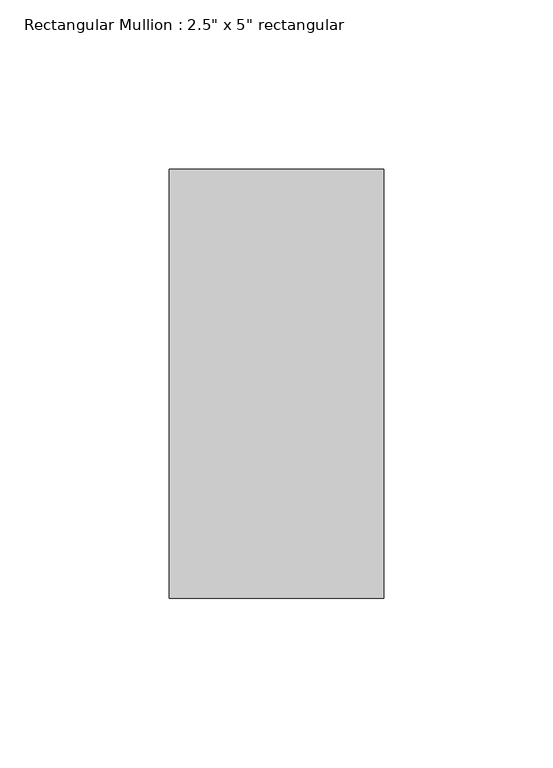
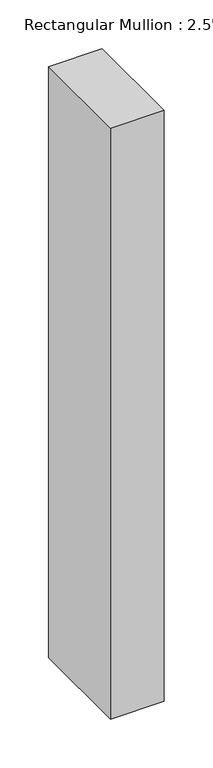
"""IFC4 building model written with IfcOpenShell, lengths in millimetres: member geometry."""

from ifc_helpers import new_model, si_unit, frame, origin, place, context, project, spatial, polyline, outline, extrude, source, transform, mapped, element, save


def member_e9f63e68(model_context):
    return source(origin(), model_context, "Body", "SweptSolid", [
        extrude(outline(polyline([(0.0, 63.5), (0.0, -63.5), (-63.5, -63.5), (-63.5, 63.5), (0.0, 63.5)])), frame((0.0, 0.0, -739.835164), z_axis=(0.0, 0.0, 1.0), x_axis=(1.0, 0.0, 0.0)), (0.0, 0.0, 1.0), 739.835164),
    ])


if __name__ == "__main__":
    model = new_model("IFC4")
    model_context = context("Model", 3, world=origin())
    ifc_project = project(units=[si_unit("LENGTHUNIT", "METRE", prefix="MILLI")], contexts=[model_context])
    site = spatial("IfcSite", under=ifc_project)
    building = spatial("IfcBuilding", under=site)
    placement = place(None, origin())
    member_shape = member_e9f63e68(model_context)
    element("IfcMember", 1, ObjectType="Rectangular Mullion : 2.5\" x 5\" rectangular", at=placement, inside=building, context=model_context, shape_type="MappedRepresentation", body=[
        mapped(member_shape, transform((0.0, 0.0, 0.0), x_axis=(1.0, 0.0, 0.0), y_axis=(0.0, 1.0, 0.0), z_axis=(0.0, 0.0, 1.0))),
    ])
    save(model, "model.ifc")

# Revit data of these elements
# Type "Rectangular Mullion : 2.5\" x 5\" rectangular"
#   built-in parameter 1007304 = 0.416667 (stored number, unit not read)
#   built-in parameter 1007301 = 0.104167 (stored number, unit not read)
#   built-in parameter 1007300 = 0.104167 (stored number, unit not read)
# Element 1 (IfcMember, "Rectangular Mullion : 2.5\" x 5\" rectangular")
#   Materials on its faces: "Aluminum"
# Materials
#   "Aluminum": class "Metal", colour RGB 247 247 247, transparency 0, Description = "Aluminum 6061", Cost = 0
